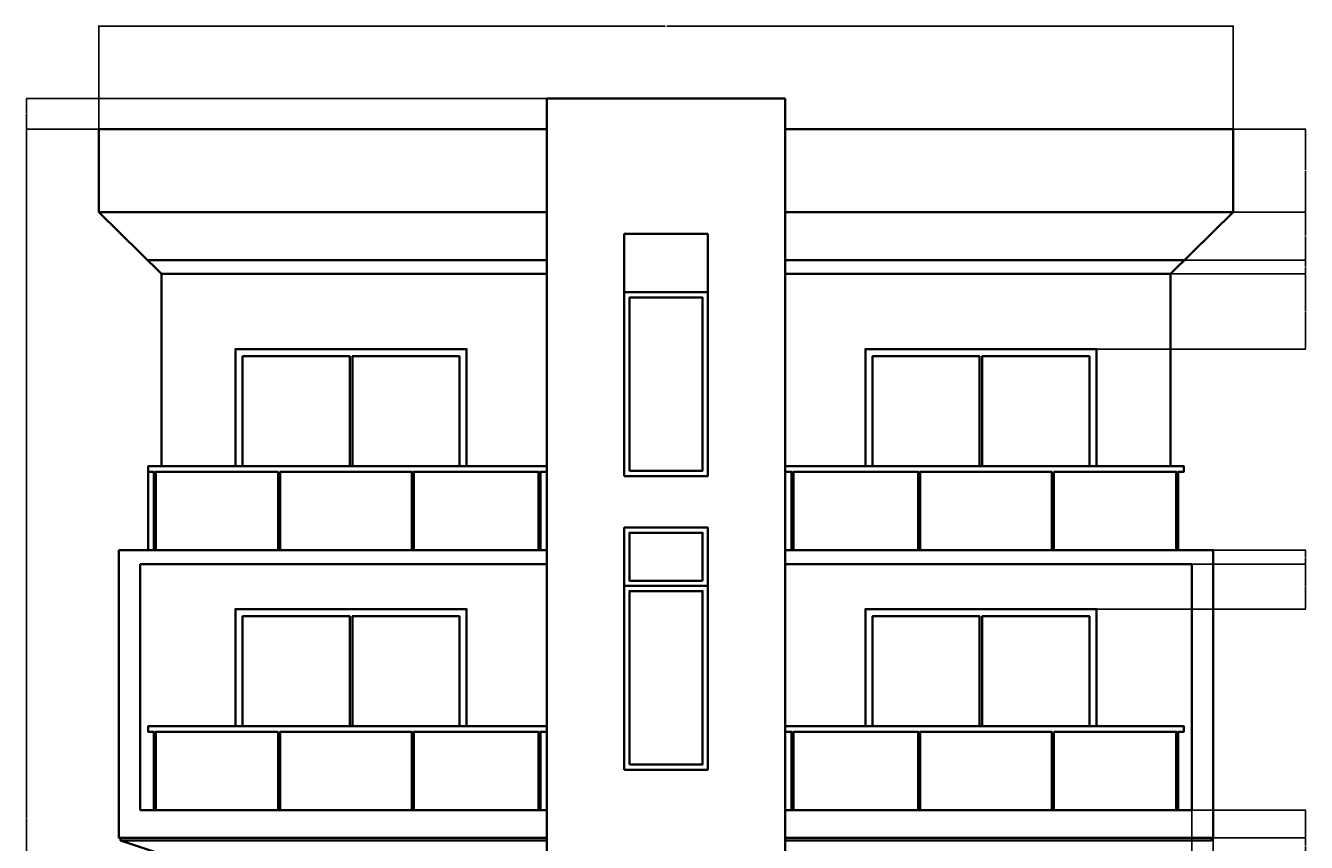
# Model space of a CAD drawing. Units: feet. Extents: x 2893 to 4112, y 897 to 1573.
# Tile 7 of 7: x 3556 to 4112, y 1218 to 1573. Entities that reach past the tile are written whole.
import ezdxf

# ---------------------------------------------------------------- set-up
doc = ezdxf.new("R2010")
doc.units = ezdxf.units.FT
for name, color, linetype, lineweight in [('A-ANNO-DIMS', 2, 'Continuous', 18), ('A-ELEV', 7, 'Continuous', 35), ('A-ELEV-PATT', 8, 'Continuous', 13)]:
    doc.layers.add(name, color=color, linetype=linetype, lineweight=lineweight)
doc.styles.get("Standard").update_dxf_attribs({"font": 'arial.ttf'})
doc.dimstyles.get("Standard").update_dxf_attribs({"dimtxt": 0.18, "dimasz": 0.18, "dimexe": 0.18, "dimexo": 0.0625, "dimgap": 0.09, "dimtad": 0, "dimtih": 1, "dimtoh": 1, "dimdec": 1, "dimzin": 0, "dimdsep": 46, "dimlunit": 3, "dimtxsty": 'Standard', "dimcen": 0.09, "dimadec": 0, "dimazin": 0, "dimtfac": 1, "dimtdec": 1, "dimtofl": 0, "dimtmove": 0, "dimatfit": 3, "dimfxl": 1, "dimtolj": 1, "dimtzin": 0, "dimarcsym": 0})

# ---------------------------------------------------------------- blocks, each defined once
blk = doc.blocks.new('*D13')
at = {"layer": 'A-ANNO-DIMS', "color": 0, "lineweight": -2, "transparency": 16777216}
for p, q in [((3587.72, 1527.95), (3587.72, 1572.84)), ((3587.9, 1572.66), (3833.75, 1572.66)), ((4080.39, 1572.66), (3834.54, 1572.66)), ((4080.57, 1527.95), (4080.57, 1572.84))]:
    blk.add_line(p, q, dxfattribs=at)
at = {"layer": 'A-ANNO-DIMS', "color": 0, "transparency": 16777216}
for points in [[(3587.9, 1572.69), (3587.9, 1572.63), (3587.72, 1572.66)], [(4080.39, 1572.69), (4080.39, 1572.63), (4080.57, 1572.66)]]:
    blk.add_solid(points, dxfattribs=at)
at = {"layer": 'Defpoints', "color": 0, "transparency": 16777216}
for p in [(4080.57, 1572.66), (3587.72, 1527.89), (4080.57, 1527.89)]:
    blk.add_point(p, dxfattribs=at)
at = {"layer": 'A-ANNO-DIMS', "color": 0, "transparency": 16777216, "insert": (3834.14, 1572.66), "char_height": 0.18, "attachment_point": 5}
blk.add_mtext('\\A1;492.8', dxfattribs=at)
blk = doc.blocks.new('*D14')
at = {"layer": 'A-ANNO-DIMS', "color": 0, "lineweight": -2, "transparency": 16777216}
for p, q in [((3587.66, 1527.89), (3556.04, 1527.89)), ((3556.22, 1527.71), (3556.22, 1228.65)), ((3556.22, 929.23), (3556.22, 1228.29)), ((3589.45, 929.05), (3556.04, 929.05))]:
    blk.add_line(p, q, dxfattribs=at)
at = {"layer": 'A-ANNO-DIMS', "color": 0, "transparency": 16777216}
for points in [[(3556.19, 1527.71), (3556.25, 1527.71), (3556.22, 1527.89)], [(3556.19, 929.23), (3556.25, 929.23), (3556.22, 929.05)]]:
    blk.add_solid(points, dxfattribs=at)
at = {"layer": 'Defpoints', "color": 0, "transparency": 16777216}
for p in [(3556.22, 1527.89), (3587.72, 1527.89), (3589.51, 929.05)]:
    blk.add_point(p, dxfattribs=at)
at = {"layer": 'A-ANNO-DIMS', "color": 0, "transparency": 16777216, "insert": (3556.22, 1228.47), "char_height": 0.18, "attachment_point": 5}
blk.add_mtext('\\A1;598.8', dxfattribs=at)
blk = doc.blocks.new('*D15')
at = {"layer": 'A-ANNO-DIMS', "color": 0, "lineweight": -2, "transparency": 16777216}
for p, q in [((3782.27, 1541.16), (3556.04, 1541.16)), ((3556.22, 1540.98), (3556.22, 1534.71)), ((3556.22, 1528.07), (3556.22, 1534.34)), ((3587.66, 1527.89), (3556.04, 1527.89))]:
    blk.add_line(p, q, dxfattribs=at)
at = {"layer": 'A-ANNO-DIMS', "color": 0, "transparency": 16777216}
for points in [[(3556.19, 1540.98), (3556.25, 1540.98), (3556.22, 1541.16)], [(3556.19, 1528.07), (3556.25, 1528.07), (3556.22, 1527.89)]]:
    blk.add_solid(points, dxfattribs=at)
at = {"layer": 'Defpoints', "color": 0, "transparency": 16777216}
for p in [(3782.33, 1541.16), (3556.22, 1527.89), (3587.72, 1527.89)]:
    blk.add_point(p, dxfattribs=at)
at = {"layer": 'A-ANNO-DIMS', "color": 0, "transparency": 16777216, "insert": (3556.22, 1534.53), "char_height": 0.18, "attachment_point": 5}
blk.add_mtext('\\A1;13.276', dxfattribs=at)
blk = doc.blocks.new('*D23')
at = {"layer": 'A-ANNO-DIMS', "color": 0, "lineweight": -2, "transparency": 16777216}
for p, q in [((4062.6, 1232.06), (4062.6, 897.37)), ((4053.45, 1212.95), (4053.45, 897.37)), ((4053.63, 897.55), (4057.7, 897.55)), ((4062.42, 897.55), (4058.35, 897.55))]:
    blk.add_line(p, q, dxfattribs=at)
at = {"layer": 'A-ANNO-DIMS', "color": 0, "transparency": 16777216}
for points in [[(4053.63, 897.58), (4053.63, 897.52), (4053.45, 897.55)], [(4062.42, 897.58), (4062.42, 897.52), (4062.6, 897.55)]]:
    blk.add_solid(points, dxfattribs=at)
at = {"layer": 'Defpoints', "color": 0, "transparency": 16777216}
for p in [(4062.6, 1232.12), (4053.45, 1213.01), (4062.6, 897.55)]:
    blk.add_point(p, dxfattribs=at)
at = {"layer": 'A-ANNO-DIMS', "color": 0, "transparency": 16777216, "insert": (4058.03, 897.55), "char_height": 0.18, "attachment_point": 5}
blk.add_mtext('\\A1;9.15', dxfattribs=at)
blk = doc.blocks.new('*D24')
at = {"layer": 'A-ANNO-DIMS', "color": 0, "lineweight": -2, "transparency": 16777216}
for p, q in [((4062.6, 1232.06), (4062.6, 897.37)), ((4071.89, 1220.03), (4071.89, 897.37)), ((4062.78, 897.55), (4066.85, 897.55)), ((4071.71, 897.55), (4067.64, 897.55))]:
    blk.add_line(p, q, dxfattribs=at)
at = {"layer": 'A-ANNO-DIMS', "color": 0, "transparency": 16777216}
for points in [[(4062.78, 897.58), (4062.78, 897.52), (4062.6, 897.55)], [(4071.71, 897.58), (4071.71, 897.52), (4071.89, 897.55)]]:
    blk.add_solid(points, dxfattribs=at)
at = {"layer": 'Defpoints', "color": 0, "transparency": 16777216}
for p in [(4062.6, 1232.12), (4071.89, 1220.09), (4071.89, 897.55)]:
    blk.add_point(p, dxfattribs=at)
at = {"layer": 'A-ANNO-DIMS', "color": 0, "transparency": 16777216, "insert": (4067.25, 897.55), "char_height": 0.18, "attachment_point": 5}
blk.add_mtext('\\A1;9.288', dxfattribs=at)
blk = doc.blocks.new('*D32')
at = {"layer": 'A-ANNO-DIMS', "color": 0, "lineweight": -2, "transparency": 16777216}
for p, q in [((4071.95, 1220.09), (4112.25, 1220.09)), ((4112.07, 1219.91), (4112.07, 1216.74)), ((4112.07, 1213.19), (4112.07, 1216.37)), ((4071.32, 1213.01), (4112.25, 1213.01))]:
    blk.add_line(p, q, dxfattribs=at)
at = {"layer": 'A-ANNO-DIMS', "color": 0, "transparency": 16777216}
for points in [[(4112.04, 1219.91), (4112.1, 1219.91), (4112.07, 1220.09)], [(4112.04, 1213.19), (4112.1, 1213.19), (4112.07, 1213.01)]]:
    blk.add_solid(points, dxfattribs=at)
at = {"layer": 'Defpoints', "color": 0, "transparency": 16777216}
for p in [(4071.89, 1220.09), (4112.07, 1220.09), (4071.26, 1213.01)]:
    blk.add_point(p, dxfattribs=at)
at = {"layer": 'A-ANNO-DIMS', "color": 0, "transparency": 16777216, "insert": (4112.07, 1216.55), "char_height": 0.18, "attachment_point": 5}
blk.add_mtext('\\A1;7.08', dxfattribs=at)
blk = doc.blocks.new('*D33')
at = {"layer": 'A-ANNO-DIMS', "color": 0, "lineweight": -2, "transparency": 16777216}
for p, q in [((4062.67, 1232.12), (4112.25, 1232.12)), ((4112.07, 1231.94), (4112.07, 1226.29)), ((4112.07, 1220.27), (4112.07, 1225.93)), ((4071.95, 1220.09), (4112.25, 1220.09))]:
    blk.add_line(p, q, dxfattribs=at)
at = {"layer": 'A-ANNO-DIMS', "color": 0, "transparency": 16777216}
for points in [[(4112.04, 1231.94), (4112.1, 1231.94), (4112.07, 1232.12)], [(4112.04, 1220.27), (4112.1, 1220.27), (4112.07, 1220.09)]]:
    blk.add_solid(points, dxfattribs=at)
at = {"layer": 'Defpoints', "color": 0, "transparency": 16777216}
for p in [(4062.6, 1232.12), (4112.07, 1232.12), (4071.89, 1220.09)]:
    blk.add_point(p, dxfattribs=at)
at = {"layer": 'A-ANNO-DIMS', "color": 0, "transparency": 16777216, "insert": (4112.07, 1226.11), "char_height": 0.18, "attachment_point": 5}
blk.add_mtext('\\A1;12.025', dxfattribs=at)
blk = doc.blocks.new('*D34')
at = {"layer": 'A-ANNO-DIMS', "color": 0, "lineweight": -2, "transparency": 16777216}
for p, q in [((4062.67, 1339.01), (4112.25, 1339.01)), ((4112.07, 1338.83), (4112.07, 1329.43)), ((4112.07, 1319.66), (4112.07, 1329.07)), ((4021.33, 1319.48), (4112.25, 1319.48))]:
    blk.add_line(p, q, dxfattribs=at)
at = {"layer": 'A-ANNO-DIMS', "color": 0, "transparency": 16777216}
for points in [[(4112.04, 1338.83), (4112.1, 1338.83), (4112.07, 1339.01)], [(4112.04, 1319.66), (4112.1, 1319.66), (4112.07, 1319.48)]]:
    blk.add_solid(points, dxfattribs=at)
at = {"layer": 'Defpoints', "color": 0, "transparency": 16777216}
for p in [(4062.6, 1339.01), (4112.07, 1339.01), (4021.27, 1319.48)]:
    blk.add_point(p, dxfattribs=at)
at = {"layer": 'A-ANNO-DIMS', "color": 0, "transparency": 16777216, "insert": (4112.07, 1329.25), "char_height": 0.18, "attachment_point": 5}
blk.add_mtext('\\A1;19.533', dxfattribs=at)
blk = doc.blocks.new('*D35')
at = {"layer": 'A-ANNO-DIMS', "color": 0, "lineweight": -2, "transparency": 16777216}
for p, q in [((4071.95, 1345.01), (4112.25, 1345.01)), ((4112.07, 1344.83), (4112.07, 1342.2)), ((4112.07, 1339.19), (4112.07, 1341.83)), ((4062.67, 1339.01), (4112.25, 1339.01))]:
    blk.add_line(p, q, dxfattribs=at)
at = {"layer": 'A-ANNO-DIMS', "color": 0, "transparency": 16777216}
for points in [[(4112.04, 1344.83), (4112.1, 1344.83), (4112.07, 1345.01)], [(4112.04, 1339.19), (4112.1, 1339.19), (4112.07, 1339.01)]]:
    blk.add_solid(points, dxfattribs=at)
at = {"layer": 'Defpoints', "color": 0, "transparency": 16777216}
for p in [(4071.89, 1345.01), (4112.07, 1345.01), (4062.6, 1339.01)]:
    blk.add_point(p, dxfattribs=at)
at = {"layer": 'A-ANNO-DIMS', "color": 0, "transparency": 16777216, "insert": (4112.07, 1342.01), "char_height": 0.18, "attachment_point": 5}
blk.add_mtext('\\A1;6', dxfattribs=at)
blk = doc.blocks.new('*D36')
at = {"layer": 'A-ANNO-DIMS', "color": 0, "lineweight": -2, "transparency": 16777216}
for p, q in [((4053.52, 1465.01), (4112.25, 1465.01)), ((4112.07, 1464.83), (4112.07, 1448.88)), ((4112.07, 1432.56), (4112.07, 1448.51)), ((4021.33, 1432.38), (4112.25, 1432.38))]:
    blk.add_line(p, q, dxfattribs=at)
at = {"layer": 'A-ANNO-DIMS', "color": 0, "transparency": 16777216}
for points in [[(4112.04, 1464.83), (4112.1, 1464.83), (4112.07, 1465.01)], [(4112.04, 1432.56), (4112.1, 1432.56), (4112.07, 1432.38)]]:
    blk.add_solid(points, dxfattribs=at)
at = {"layer": 'Defpoints', "color": 0, "transparency": 16777216}
for p in [(4053.45, 1465.01), (4112.07, 1465.01), (4021.27, 1432.38)]:
    blk.add_point(p, dxfattribs=at)
at = {"layer": 'A-ANNO-DIMS', "color": 0, "transparency": 16777216, "insert": (4112.07, 1448.7), "char_height": 0.18, "attachment_point": 5}
blk.add_mtext('\\A1;32.64', dxfattribs=at)
blk = doc.blocks.new('*D37')
at = {"layer": 'A-ANNO-DIMS', "color": 0, "lineweight": -2, "transparency": 16777216}
for p, q in [((4059.57, 1471.01), (4112.25, 1471.01)), ((4112.07, 1470.83), (4112.07, 1468.2)), ((4053.52, 1465.01), (4112.25, 1465.01)), ((4112.07, 1465.19), (4112.07, 1467.83))]:
    blk.add_line(p, q, dxfattribs=at)
at = {"layer": 'A-ANNO-DIMS', "color": 0, "transparency": 16777216}
for points in [[(4112.04, 1470.83), (4112.1, 1470.83), (4112.07, 1471.01)], [(4112.04, 1465.19), (4112.1, 1465.19), (4112.07, 1465.01)]]:
    blk.add_solid(points, dxfattribs=at)
at = {"layer": 'Defpoints', "color": 0, "transparency": 16777216}
for p in [(4059.51, 1471.01), (4112.07, 1471.01), (4053.45, 1465.01)]:
    blk.add_point(p, dxfattribs=at)
at = {"layer": 'A-ANNO-DIMS', "color": 0, "transparency": 16777216, "insert": (4112.07, 1468.01), "char_height": 0.18, "attachment_point": 5}
blk.add_mtext('\\A1;6', dxfattribs=at)
blk = doc.blocks.new('*D38')
at = {"layer": 'A-ANNO-DIMS', "color": 0, "lineweight": -2, "transparency": 16777216}
for p, q in [((4080.63, 1491.89), (4112.25, 1491.89)), ((4112.07, 1491.71), (4112.07, 1481.63)), ((4112.07, 1471.19), (4112.07, 1481.27)), ((4059.57, 1471.01), (4112.25, 1471.01))]:
    blk.add_line(p, q, dxfattribs=at)
at = {"layer": 'A-ANNO-DIMS', "color": 0, "transparency": 16777216}
for points in [[(4112.04, 1491.71), (4112.1, 1491.71), (4112.07, 1491.89)], [(4112.04, 1471.19), (4112.1, 1471.19), (4112.07, 1471.01)]]:
    blk.add_solid(points, dxfattribs=at)
at = {"layer": 'Defpoints', "color": 0, "transparency": 16777216}
for p in [(4080.57, 1491.89), (4112.07, 1491.89), (4059.51, 1471.01)]:
    blk.add_point(p, dxfattribs=at)
at = {"layer": 'A-ANNO-DIMS', "color": 0, "transparency": 16777216, "insert": (4112.07, 1481.45), "char_height": 0.18, "attachment_point": 5}
blk.add_mtext('\\A1;20.875', dxfattribs=at)
blk = doc.blocks.new('*D39')
at = {"layer": 'A-ANNO-DIMS', "color": 0, "lineweight": -2, "transparency": 16777216}
for p, q in [((4080.63, 1527.89), (4112.25, 1527.89)), ((4112.07, 1527.71), (4112.07, 1510.07)), ((4112.07, 1492.07), (4112.07, 1509.71)), ((4080.63, 1491.89), (4112.25, 1491.89))]:
    blk.add_line(p, q, dxfattribs=at)
at = {"layer": 'A-ANNO-DIMS', "color": 0, "transparency": 16777216}
for points in [[(4112.04, 1527.71), (4112.1, 1527.71), (4112.07, 1527.89)], [(4112.04, 1492.07), (4112.1, 1492.07), (4112.07, 1491.89)]]:
    blk.add_solid(points, dxfattribs=at)
at = {"layer": 'Defpoints', "color": 0, "transparency": 16777216}
for p in [(4080.57, 1527.89), (4112.07, 1527.89), (4080.57, 1491.89)]:
    blk.add_point(p, dxfattribs=at)
at = {"layer": 'A-ANNO-DIMS', "color": 0, "transparency": 16777216, "insert": (4112.07, 1509.89), "char_height": 0.18, "attachment_point": 5}
blk.add_mtext('\\A1;36', dxfattribs=at)

msp = doc.modelspace()

# ---------------------------------------------------------------- hatches: boundary and pattern name
at = {"layer": 'A-ELEV-PATT'}
h = msp.add_hatch(color=256, dxfattribs=at)
h.dxf.hatch_style = 1
h.paths.add_polyline_path([(3818.239, 1480.0922), (3850.0494, 1480.0922), (3850.0494, 1459.3019), (3818.239, 1459.3019)], flags=16)
h.paths.add_polyline_path([(3609.0791, 1345.0143), (3609.0791, 1381.4641), (3647.022, 1381.4641), (3647.022, 1432.3761), (3747.5019, 1432.3761), (3747.5019, 1381.4641), (3782.3275, 1381.4641), (3782.3275, 1345.0143)])
h.paths.add_polyline_path([(3609.0791, 1345.0143), (3609.0791, 1381.4641), (3647.022, 1381.4641), (3647.022, 1432.3761), (3747.5019, 1432.3761), (3747.5019, 1381.4641), (3782.3275, 1381.4641), (3782.3275, 1345.0143)])
h.paths.add_polyline_path([(3782.3275, 1232.1197), (3611.5098, 1232.1197), (3611.5098, 1266.188), (3609.0791, 1266.188), (3609.0791, 1268.5695), (3647.022, 1268.5695), (3647.022, 1319.4814), (3747.5019, 1319.4814), (3747.5019, 1268.5695), (3782.3275, 1268.5695)])
h.paths.add_polyline_path([(3782.3275, 1232.1197), (3611.5098, 1232.1197), (3611.5098, 1266.188), (3609.0791, 1266.188), (3609.0791, 1268.5695), (3647.022, 1268.5695), (3647.022, 1319.4814), (3747.5019, 1319.4814), (3747.5019, 1268.5695), (3782.3275, 1268.5695)])
h.paths.add_polyline_path([(3850.0494, 1480.0922), (3850.0494, 1459.3019), (3818.239, 1459.3019), (3818.239, 1480.0922)])

# ---------------------------------------------------------------- linework, layer by layer
at = {"layer": 'A-ELEV'}
for p, q in [((3782.3275, 967.0143), (3782.3275, 1541.1646)), ((3782.3275, 1541.1646), (3885.9608, 1541.1646)), ((3885.9608, 967.0143), (3885.9608, 1541.1646)), ((3587.7226, 1491.889), (3587.7226, 1527.889)), ((3587.7226, 1527.889), (3782.3275, 1527.889)), ((3885.9608, 1527.889), (4080.5657, 1527.889)), ((4080.5657, 1491.889), (4080.5657, 1527.889)), ((3614.8353, 1465.0143), (3587.7226, 1491.889)), ((3587.7226, 1491.889), (3782.3275, 1491.889)), ((4080.5657, 1491.889), (3885.9608, 1491.889)), ((4053.4531, 1465.0143), (4080.5657, 1491.889)), ((3782.3275, 1471.0143), (3608.7821, 1471.0143)), ((4059.5062, 1471.0143), (3885.9608, 1471.0143)), ((3614.8353, 1465.0143), (3782.3275, 1465.0143)), ((3614.8353, 1381.4641), (3614.8353, 1465.0143)), ((3614.8353, 1465.0143), (3614.8353, 1381.4641)), ((3885.9608, 1465.0143), (4053.4531, 1465.0143)), ((4053.4531, 1465.0143), (4053.4531, 1381.4641)), ((3609.0791, 1381.4641), (3609.0791, 1345.0143)), ((3782.3275, 1345.0143), (3596.3966, 1345.0143)), ((3596.3966, 1220.0947), (3596.3966, 1345.0143)), ((4071.8918, 1345.0143), (3885.9608, 1345.0143)), ((4071.8918, 1220.0947), (4071.8918, 1345.0143)), ((3605.6845, 1339.0143), (3782.3275, 1339.0143)), ((3885.9608, 1339.0143), (4062.6038, 1339.0143)), ((3597.0307, 1220.0947), (3596.3966, 1220.0947)), ((3597.0307, 1219.0143), (3597.0307, 1220.0947)), ((3782.3275, 1219.0143), (3597.0307, 1219.0143)), ((3614.8353, 1213.0143), (3597.0307, 1219.0143)), ((4071.2577, 1219.0143), (3885.9608, 1219.0143))]:
    msp.add_line(p, q, dxfattribs=at)
for points in [[(3852.3189, 1457.0324), (3815.9695, 1457.0324), (3815.9695, 1482.3616), (3852.3189, 1482.3616)], [(3815.9695, 1377.2236), (3852.3189, 1377.2236), (3852.3189, 1457.0324), (3815.9695, 1457.0324)], [(3818.239, 1379.4931), (3850.0494, 1379.4931), (3850.0494, 1454.7629), (3818.239, 1454.7629)], [(3747.5019, 1381.4641), (3647.022, 1381.4641), (3647.022, 1432.3761), (3747.5019, 1432.3761)], [(3920.7865, 1381.4641), (4021.2664, 1381.4641), (4021.2664, 1432.3761), (3920.7865, 1432.3761)], [(3665.6357, 1379.0826), (3612.3836, 1379.0826), (3612.3836, 1345.0143), (3611.5098, 1345.0143), (3611.5098, 1379.0826), (3609.0791, 1379.0826), (3609.0791, 1381.4641), (3782.3275, 1381.4641), (3782.3275, 1379.0826), (3779.5608, 1379.0826), (3779.5608, 1345.0143), (3778.687, 1345.0143), (3778.687, 1379.0826), (3724.5465, 1379.0826), (3724.5465, 1345.0143), (3723.6728, 1345.0143), (3723.6728, 1379.0826), (3666.5095, 1379.0826), (3666.5095, 1345.0143), (3665.6357, 1345.0143)], [(4002.6527, 1379.0826), (4055.9048, 1379.0826), (4055.9048, 1345.0143), (4056.7785, 1345.0143), (4056.7785, 1379.0826), (4059.2093, 1379.0826), (4059.2093, 1381.4641), (3885.9608, 1381.4641), (3885.9608, 1379.0826), (3888.7276, 1379.0826), (3888.7276, 1345.0143), (3889.6014, 1345.0143), (3889.6014, 1379.0826), (3943.7418, 1379.0826), (3943.7418, 1345.0143), (3944.6156, 1345.0143), (3944.6156, 1379.0826), (4001.7789, 1379.0826), (4001.7789, 1345.0143), (4002.6527, 1345.0143)], [(3852.3189, 1329.5145), (3815.9695, 1329.5145), (3815.9695, 1354.8437), (3852.3189, 1354.8437)], [(3850.0494, 1331.784), (3818.239, 1331.784), (3818.239, 1352.5742), (3850.0494, 1352.5742)], [(3815.9695, 1249.7057), (3852.3189, 1249.7057), (3852.3189, 1329.5145), (3815.9695, 1329.5145)], [(3818.239, 1251.9752), (3850.0494, 1251.9752), (3850.0494, 1327.245), (3818.239, 1327.245)], [(3747.5019, 1268.5695), (3647.022, 1268.5695), (3647.022, 1319.4814), (3747.5019, 1319.4814)], [(3920.7865, 1268.5695), (4021.2664, 1268.5695), (4021.2664, 1319.4814), (3920.7865, 1319.4814)], [(3665.6357, 1266.188), (3612.3836, 1266.188), (3612.3836, 1232.1197), (3611.5098, 1232.1197), (3611.5098, 1266.188), (3609.0791, 1266.188), (3609.0791, 1268.5695), (3782.3275, 1268.5695), (3782.3275, 1266.188), (3779.5608, 1266.188), (3779.5608, 1232.1197), (3778.687, 1232.1197), (3778.687, 1266.188), (3724.5465, 1266.188), (3724.5465, 1232.1197), (3723.6728, 1232.1197), (3723.6728, 1266.188), (3666.5095, 1266.188), (3666.5095, 1232.1197), (3665.6357, 1232.1197)], [(4002.6527, 1266.188), (4055.9048, 1266.188), (4055.9048, 1232.1197), (4056.7785, 1232.1197), (4056.7785, 1266.188), (4059.2093, 1266.188), (4059.2093, 1268.5695), (3885.9608, 1268.5695), (3885.9608, 1266.188), (3888.7276, 1266.188), (3888.7276, 1232.1197), (3889.6014, 1232.1197), (3889.6014, 1266.188), (3943.7418, 1266.188), (3943.7418, 1232.1197), (3944.6156, 1232.1197), (3944.6156, 1266.188), (4001.7789, 1266.188), (4001.7789, 1232.1197), (4002.6527, 1232.1197)], [(3782.3275, 1219.0143), (3597.0307, 1219.0143), (3597.0307, 1220.0947), (3782.3275, 1220.0947)], [(3885.9608, 1219.0143), (4071.2577, 1219.0143), (4071.2577, 1220.0947), (3885.9608, 1220.0947)]]:
    msp.add_lwpolyline(points, close=True, dxfattribs=at)
for points in [[(3744.3518, 1381.4641), (3744.3518, 1429.226), (3697.8342, 1429.226), (3697.8342, 1381.4641), (3696.6897, 1381.4641), (3696.6897, 1429.226), (3650.1721, 1429.226), (3650.1721, 1381.4641)], [(3923.9365, 1381.4641), (3923.9365, 1429.226), (3970.4542, 1429.226), (3970.4542, 1381.4641), (3971.5986, 1381.4641), (3971.5986, 1429.226), (4018.1163, 1429.226), (4018.1163, 1381.4641)], [(3596.3966, 1232.1197), (3596.3966, 1345.0143)], [(4062.6038, 1220.0947), (4071.8918, 1220.0947), (4071.8918, 1345.0143)], [(3605.6845, 1339.0143), (3605.6845, 1232.1197)], [(4062.6038, 1339.0143), (4062.6038, 1232.1197)], [(3744.3518, 1268.5695), (3744.3518, 1316.3314), (3697.8342, 1316.3314), (3697.8342, 1268.5695), (3696.6897, 1268.5695), (3696.6897, 1316.3314), (3650.1721, 1316.3314), (3650.1721, 1268.5695)], [(3923.9365, 1268.5695), (3923.9365, 1316.3314), (3970.4542, 1316.3314), (3970.4542, 1268.5695), (3971.5986, 1268.5695), (3971.5986, 1316.3314), (4018.1163, 1316.3314), (4018.1163, 1268.5695)], [(3596.3966, 1232.1197), (3596.3966, 1220.0947), (3782.3275, 1220.0947), (3782.3275, 1232.1197), (3605.6845, 1232.1197)], [(4071.8918, 1232.1197), (4071.8918, 1220.0947), (3885.9608, 1220.0947), (3885.9608, 1232.1197), (4062.6038, 1232.1197)]]:
    msp.add_lwpolyline(points, dxfattribs=at)

# ---------------------------------------------------------------- dimensions: what is measured, and where the dimension line sits
at = {"layer": 'A-ANNO-DIMS'}
for base, p1, p2, override, picture, middle in [((4080.5657, 1572.6646), (3587.7226, 1527.889), (4080.5657, 1527.889), {"dimdec": 1, "dimlfac": 1, "dimrnd": 0, "dimzin": 0, "dimdsep": 46, "dimlunit": 2}, '*D13', (3834.1442, 1572.6646)), ((4062.6038, 897.5499), (4053.4531, 1213.0143), (4062.6038, 1232.1197), {"dimdec": 2, "dimlfac": 1, "dimrnd": 0, "dimzin": 0, "dimdsep": 46, "dimlunit": 2}, '*D23', (4058.0285, 897.5499)), ((4071.8918, 897.5499), (4062.6038, 1232.1197), (4071.8918, 1220.0947), {"dimdec": 3, "dimlfac": 1, "dimrnd": 0, "dimzin": 0, "dimdsep": 46, "dimlunit": 2}, '*D24', (4067.2478, 897.5499))]:
    dim = msp.add_linear_dim(base=base, p1=p1, p2=p2, dimstyle='Standard', override=override, dxfattribs=at)
    dim.commit()
    dim.dimension.update_dxf_attribs({"geometry": picture, "text_midpoint": middle})
for base, p1, p2, override, picture, middle in [((3556.2226, 1527.889), (3782.3275, 1541.1646), (3587.7226, 1527.889), {"dimdec": 3, "dimlfac": 1, "dimrnd": 0, "dimzin": 0, "dimdsep": 46, "dimlunit": 2}, '*D15', (3556.2226, 1534.5268)), ((3556.2226, 1527.889), (3589.5092, 929.0499), (3587.7226, 1527.889), {"dimdec": 1, "dimlfac": 1, "dimrnd": 0, "dimzin": 0, "dimdsep": 46, "dimlunit": 2}, '*D14', (3556.2226, 1228.4695)), ((4112.0657, 1527.889), (4080.5657, 1491.889), (4080.5657, 1527.889), {"dimdec": 0, "dimlfac": 1, "dimrnd": 0, "dimzin": 0, "dimdsep": 46, "dimlunit": 2}, '*D39', (4112.0657, 1509.889)), ((4112.0657, 1491.889), (4059.5062, 1471.0143), (4080.5657, 1491.889), {"dimdec": 3, "dimlfac": 1, "dimrnd": 0, "dimzin": 0, "dimdsep": 46, "dimlunit": 2}, '*D38', (4112.0657, 1481.4517)), ((4112.0657, 1471.0143), (4053.4531, 1465.0143), (4059.5062, 1471.0143), {"dimdec": 0, "dimlfac": 1, "dimrnd": 0, "dimzin": 0, "dimdsep": 46, "dimlunit": 2}, '*D37', (4112.0657, 1468.0143)), ((4112.0657, 1465.0143), (4021.2664, 1432.3761), (4053.4531, 1465.0143), {"dimdec": 2, "dimlfac": 1, "dimrnd": 0, "dimzin": 0, "dimdsep": 46, "dimlunit": 2}, '*D36', (4112.0657, 1448.6952)), ((4112.0657, 1345.0143), (4062.6038, 1339.0143), (4071.8918, 1345.0143), {"dimdec": 0, "dimlfac": 1, "dimrnd": 0, "dimzin": 0, "dimdsep": 46, "dimlunit": 2}, '*D35', (4112.0657, 1342.0143)), ((4112.0657, 1339.0143), (4021.2664, 1319.4814), (4062.6038, 1339.0143), {"dimdec": 3, "dimlfac": 1, "dimrnd": 0, "dimzin": 0, "dimdsep": 46, "dimlunit": 2}, '*D34', (4112.0657, 1329.2479)), ((4112.0657, 1232.1197), (4071.8918, 1220.0947), (4062.6038, 1232.1197), {"dimdec": 3, "dimlfac": 1, "dimrnd": 0, "dimzin": 0, "dimdsep": 46, "dimlunit": 2}, '*D33', (4112.0657, 1226.1072)), ((4112.0657, 1220.0947), (4071.2577, 1213.0143), (4071.8918, 1220.0947), {"dimdec": 2, "dimlfac": 1, "dimrnd": 0, "dimzin": 0, "dimdsep": 46, "dimlunit": 2}, '*D32', (4112.0657, 1216.5545))]:
    dim = msp.add_linear_dim(base=base, p1=p1, p2=p2, angle=90, dimstyle='Standard', override=override, dxfattribs=at)
    dim.commit()
    dim.dimension.update_dxf_attribs({"geometry": picture, "text_midpoint": middle})

doc.saveas('drawing.dxf')
